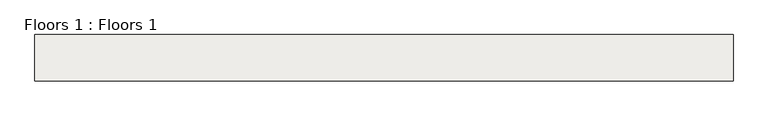
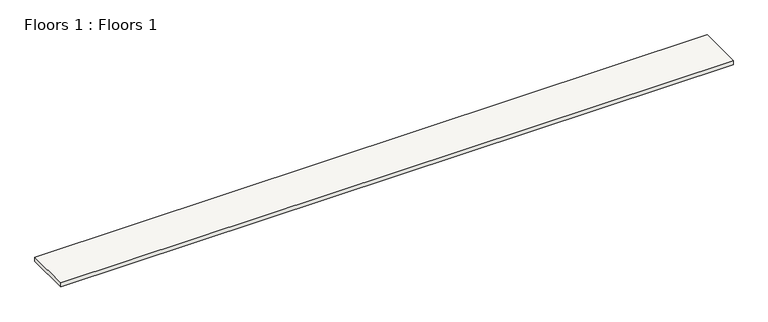
"""IFC4 building model written with IfcOpenShell, lengths in millimetres: slab geometry, Floors 1 : Floors 1."""

from ifc_helpers import new_model, si_unit, frame, origin, place, context, project, spatial, polyline, outline, extrude, source, transform, mapped, element, save


def floors_1_floors_1_86c0a0b5(model_context):
    return source(origin(), model_context, "Body", "SweptSolid", [
        extrude(outline(polyline([(41445.3647012, -8313.0706022), (41445.3647012, -10141.8706022), (14013.3647012, -10141.8706022), (14013.3647012, -8313.0706022), (41445.3647012, -8313.0706022)])), frame((0.0, 0.0, -304.8), z_axis=(0.0, 0.0, 1.0), x_axis=(1.0, 0.0, 0.0)), (0.0, 0.0, 1.0), 172.7176062),
    ])


if __name__ == "__main__":
    model = new_model("IFC4")
    model_context = context("Model", 3, world=origin())
    ifc_project = project(units=[si_unit("LENGTHUNIT", "METRE", prefix="MILLI")], contexts=[model_context])
    site = spatial("IfcSite", under=ifc_project)
    building = spatial("IfcBuilding", under=site)
    placement = place(None, origin())
    floors_1_floors_1_shape = floors_1_floors_1_86c0a0b5(model_context)
    element("IfcSlab", 1, ObjectType="Floors 1 : Floors 1", at=placement, inside=building, context=model_context, shape_type="MappedRepresentation", body=[
        mapped(floors_1_floors_1_shape, transform((0.0, 0.0, 0.0), x_axis=(1.0, 0.0, 0.0), y_axis=(0.0, 1.0, 0.0), z_axis=(0.0, 0.0, 1.0))),
    ])
    save(model, "model.ifc")

# Revit data of these elements
# Element 1 (IfcSlab, "Floors 1 : Floors 1")
#   Materials on its faces: "Concrete, Cast-in-Place gray"
# Materials
#   "Concrete, Cast-in-Place gray": class "Concrete", colour RGB 192 192 192, transparency 0, Description = "Cast-in-place concrete", Cost = 0
